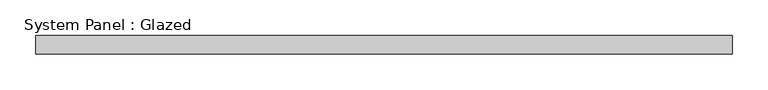
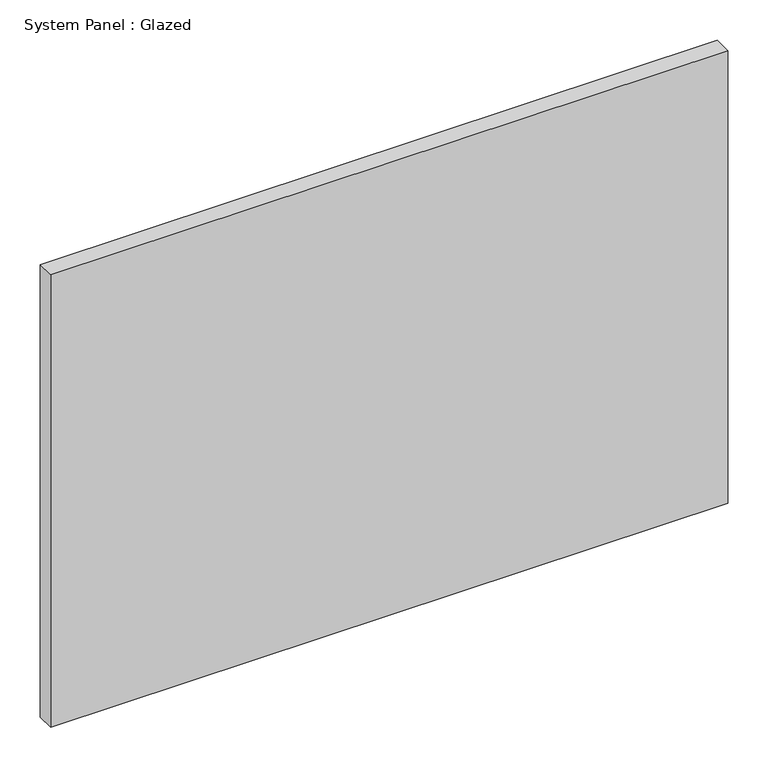
"""IFC4 building model written with IfcOpenShell, lengths in millimetres: plate geometry, System Panel : Glazed."""

from ifc_helpers import new_model, si_unit, origin, origin_with_axes, place, context, project, spatial, polyline, outline, extrude, source, transform, mapped, element, save


def system_panel_glazed_a4f4dc30(model_context):
    return source(origin(), model_context, "Body", "SweptSolid", [
        extrude(outline(polyline([(484.7166667, 19.05), (-484.7166667, 19.05), (-484.7166667, 44.45), (484.7166667, 44.45), (484.7166667, 19.05)])), origin_with_axes(), (0.0, 0.0, 1.0), 684.9785678),
    ])


if __name__ == "__main__":
    model = new_model("IFC4")
    model_context = context("Model", 3, world=origin())
    ifc_project = project(units=[si_unit("LENGTHUNIT", "METRE", prefix="MILLI")], contexts=[model_context])
    site = spatial("IfcSite", under=ifc_project)
    building = spatial("IfcBuilding", under=site)
    placement = place(None, origin())
    system_panel_glazed_shape = system_panel_glazed_a4f4dc30(model_context)
    element("IfcPlate", 1, ObjectType="System Panel : Glazed", at=placement, inside=building, context=model_context, shape_type="MappedRepresentation", body=[
        mapped(system_panel_glazed_shape, transform((0.0, 0.0, 0.0), x_axis=(1.0, 0.0, 0.0), y_axis=(0.0, 1.0, 0.0), z_axis=(0.0, 0.0, 1.0))),
    ])
    save(model, "model.ifc")

# Revit data of these elements
# Type "System Panel : Glazed"
#   Construction Type Id = "GSP4R"
#   Analytic Construction = "1/8 in Pilkington single glazing"
#   Visual Light Transmittance = 0.9
#   Solar Heat Gain Coefficient = 0.86
#   Heat Transfer Coefficient (U) = 1.18115 BTU/(h·ft²·°F)
#   Define Thermal Properties by = 1
# Element 1 (IfcPlate, "System Panel : Glazed")
#   Materials on its faces: "Glass"
# Materials
#   "Glass": class "Glass", colour RGB 0 128 192, transparency 0.75, Description = "Soda Lime Glass", Cost = 0
